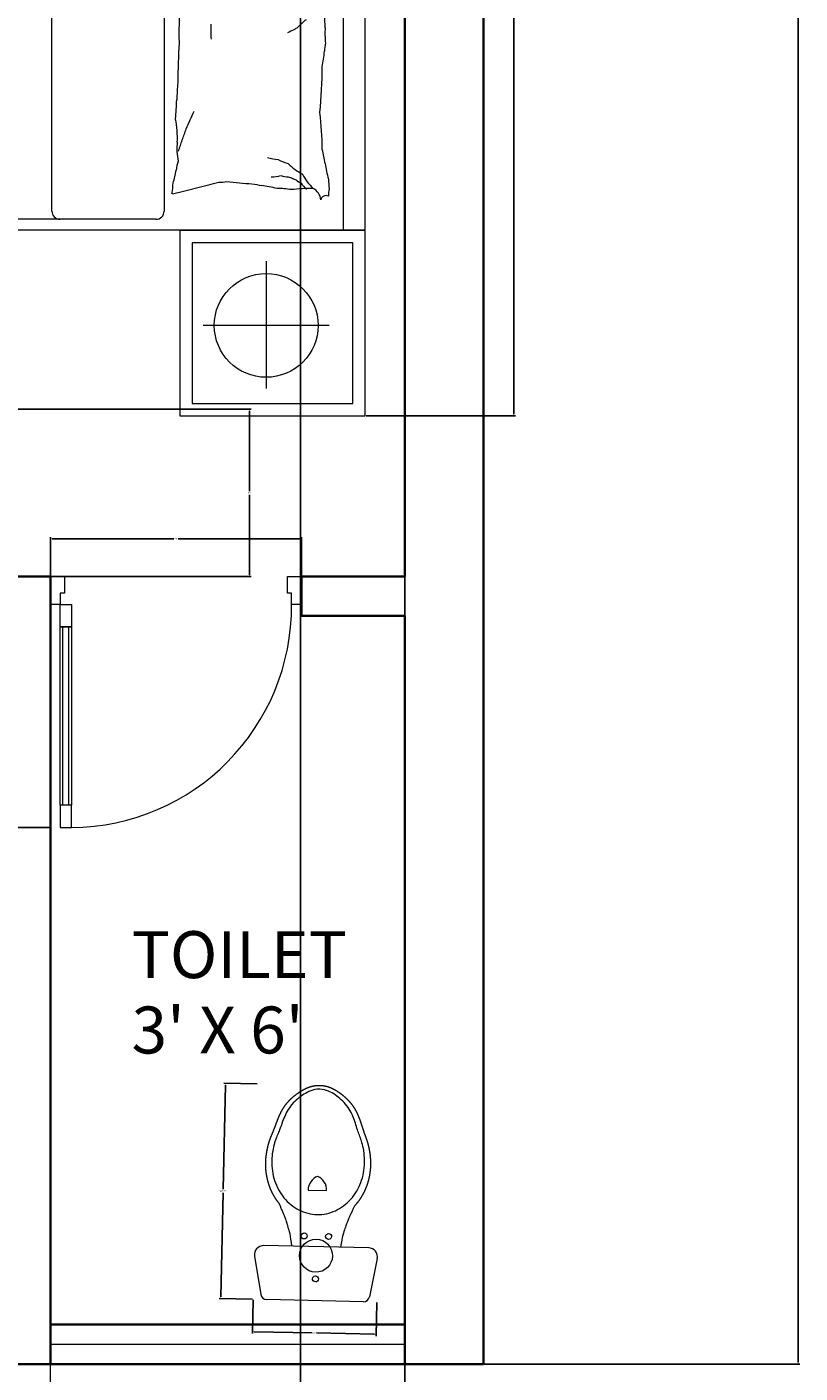
# Model space of a CAD drawing. Units: feet. Extents: x 1993 to 2298, y 2938 to 3641.
# Tile 4 of 11: x 2219 to 2298, y 3008 to 3144. Entities that reach past the tile are written whole.
import ezdxf

# ---------------------------------------------------------------- set-up
doc = ezdxf.new("R2010")
doc.units = ezdxf.units.FT
doc.linetypes.add('ACAD_ISO02W100', pattern=[15, 12, -3])
for name, color, linetype, lineweight in [('A-ANNO-DIMS', 2, 'Continuous', 18), ('A-AREA-IDEN', 7, 'Continuous', 18), ('A-DOOR', 3, 'Continuous', 18), ('A-FLOR-FIXT', 9, 'Continuous', 18), ('A-GLAZ', 4, 'Continuous', 13), ('DWV_RED', 7, 'Continuous', 0), ('furniture', 8, 'Continuous', 18), ('SUNSHADES', 4, 'ACAD_ISO02W100', 13), ('WAL', 7, 'Continuous', 35)]:
    doc.layers.add(name, color=color, linetype=linetype, lineweight=lineweight)
doc.styles.add('DIM_FONT', font='SIMPLEX.shx', dxfattribs={"width": 0.8})
doc.styles.get("Standard").update_dxf_attribs({"font": 'arial.ttf'})
doc.dimstyles.get("Standard").update_dxf_attribs({"dimtxt": 0.18, "dimasz": 0.18, "dimexe": 0.18, "dimexo": 0.0625, "dimgap": 0.09, "dimtad": 0, "dimtih": 1, "dimtoh": 1, "dimdec": 4, "dimzin": 0, "dimdsep": 46, "dimtxsty": 'Standard', "dimcen": 0.09, "dimadec": 0, "dimazin": 0, "dimtfac": 1, "dimtdec": 4, "dimtofl": 0, "dimtmove": 0, "dimatfit": 3, "dimfxl": 1, "dimtolj": 1, "dimtzin": 0, "dimarcsym": 0})

# ---------------------------------------------------------------- blocks, each defined once
blk = doc.blocks.new('A$C184E58E8')
for points in [[(825, 900), (825, 820), (865, 820), (865, 900)], [(825, 180), (825, 820), (865, 820), (865, 180)], [(835, 180), (835, 820), (855, 820), (855, 180)], [(825, 100), (825, 180), (865, 180), (865, 100)], [(35, 100), (35, 60), (50, 60), (50, 50), (50, 0), (0, 0), (0, 100)], [(865, 100), (900, 100), (900, 0), (850, 0), (850, 50), (850, 60), (865, 60)]]:
    blk.add_lwpolyline(points, close=True)
blk.add_arc((830, 105), 795, 90.3603, 180.3603)
blk = doc.blocks.new('A$C79766A75')
for p, q in [((1.9506, 2), (0.4506, 2)), ((1.9506, 0), (1.9506, 2)), ((2.402, 1.9999), (1.952, 1.9999)), ((1.952, 1.9999), (1.952, 1.5499)), ((2.402, 1.5499), (2.402, 1.9999)), ((2.372, 1.9699), (1.982, 1.9699)), ((1.982, 1.9699), (1.982, 1.5799)), ((2.372, 1.5799), (2.372, 1.9699)), ((1.9506, 1.9476), (0.4506, 1.9476)), ((2.1824, 1.9125), (2.1824, 1.6061)), ((2.0263, 1.7595), (2.3354, 1.7595)), ((1.8553, 1.5617), (1.8346, 1.6443)), ((1.982, 1.5799), (2.372, 1.5799)), ((1.8628, 1.5317), (1.8553, 1.5617)), ((1.952, 1.5499), (2.402, 1.5499)), ((1.0972, 1.5115), (1.9048, 1.5115)), ((1.9248, 1.4915), (1.9248, 0.0322)), ((1.9048, 1.2389), (1.0354, 1.2389))]:
    blk.add_line(p, q)
blk.add_circle((2.1824, 1.7595), 0.126)
for centre, radius, start, end in [((1.4683, 1.0293), 0.8732, 90.5757, 94.8018), ((1.4724, 2.1919), 0.2897, 267.4614, 274.8018), ((1.5236, 2.0532), 0.1524, 259.8101, 267.4614), ((1.4607, 1.3747), 0.5293, 79.8101, 83.9133), ((1.821, 1.6625), 0.2422, 97.5469, 105.744), ((1.7444, 2.2041), 0.3048, 278.4372, 285.744), ((1.8271, 2.0719), 0.1611, 270, 278.4372), ((1.8684, 2.0011), 0.0904, 258.7276, 270), ((1.8802, 1.9049), 0.0131, 153.4195, 258.7276), ((1.5543, 0.8466), 1.049, 83.9133, 90), ((1.7552, 1.2129), 0.6827, 90, 97.5469), ((1.7511, 1.9723), 0.1399, 297.2036, 314.9024), ((1.8802, 1.8579), 0.0342, 94.4002, 153.4195), ((2.3416, 1.8735), 0.4918, 180, 186.2324), ((1.615, 1.9982), 0.2252, 219.0349, 226.1885), ((1.5025, 1.8591), 0.0493, 208.3168, 219.0349), ((1.6908, 1.9123), 0.1399, 314.9024, 332.6012), ((1.6887, 1.8881), 0.1511, 334.6449, 338.1851), ((1.7896, 1.8667), 0.0526, 318.5571, 334.6449), ((1.784, 1.9167), 0.0899, 306.2641, 318.5571), ((1.6484, 1.9062), 0.2002, 203.0028, 208.3168), ((1.6554, 1.8529), 0.1399, 332.6012, 343.485), ((1.7653, 1.8132), 0.0562, 341.2201, 0), ((1.6307, 1.8895), 0.2056, 338.1851, 341.2201), ((2.0538, 1.7858), 0.204, 170.3156, 180), ((1.6404, 1.8023), 0.1399, 343.485, 354.3689), ((1.73, 1.7719), 0.0915, 0, 14.6851), ((2.7119, 1.5994), 0.882, 167.8016, 170.3156), ((1.5284, 1.792), 0.3171, 347.8016, 351.9949), ((1.1803, 1.7556), 0.6588, 351.9949, 357.3351), ((1.767, 1.6474), 0.0677, 357.3351, 14.0452), ((1.4679, 1.8969), 0.2721, 266.4448, 274.0828), ((1.3675, 0.9067), 0.7387, 64.6889, 66.5156), ((1.4107, 0.888), 0.7387, 66.5156, 68.3423), ((1.4677, 7.2662), 5.7185, 269.0296, 270.2865), ((1.6493, 4.9065), 3.3622, 267.3904, 269.0296), ((1.6903, 2.7573), 1.2165, 265.3824, 267.3904), ((1.5676, 0.139), 1.4048, 85.3824, 87.2509), ((1.7268, 1.3138), 0.2301, 87.2509, 101.5586), ((1.4594, 0.8688), 0.7387, 68.3423, 70.572), ((1.5136, 0.8497), 0.7387, 70.572, 72.8018), ((1.7541, 1.6886), 0.1459, 263.5659, 281.5586), ((1.8192, 1.6599), 0.1197, 252.6136, 263.5659), ((1.7679, 1.3144), 0.2297, 72.6136, 80.5159), ((1.8172, 1.2635), 0.2708, 80.5159, 85.9171), ((1.8627, 1.5308), 0.000917, 85.9171, 194.0449), ((1.9048, 1.4915), 0.02, 0, 90), ((1.9048, 1.2589), 0.02, 270, 0)]:
    blk.add_arc(centre, radius, start, end)
at = {"style": 'DIM_FONT', "text_generation_flag": 4, "width": 0.8, "flags": 9}
for tag in ['XSIZE', 'YSIZE']:
    blk.add_attdef(tag, (1.9506, 2), '', height=0.0005, rotation=180, dxfattribs=at)
blk = doc.blocks.new('A$C6F4D5F33')
at = {"layer": 'DWV_RED'}
for p, q in [((142.3, 403.6), (16.1, 380.5)), ((0, 42.9), (0, 361.2)), ((177.2, 29.5), (177.2, 374.6)), ((447.9, 353.8), (439.5, 353.3)), ((456.2, 354), (447.9, 353.8)), ((464.5, 353.9), (456.2, 354)), ((472.6, 353.4), (464.5, 353.9)), ((335.6, 311.2), (329.7, 305.8)), ((341.8, 316.3), (335.6, 311.2)), ((348.2, 321), (341.8, 316.3)), ((354.9, 325.5), (348.2, 321)), ((361.8, 329.7), (354.9, 325.5)), ((368.9, 333.5), (361.8, 329.7)), ((376.2, 337), (368.9, 333.5)), ((383.7, 340.2), (376.2, 337)), ((391.3, 343.1), (383.7, 340.2)), ((399.1, 345.6), (391.3, 343.1)), ((407, 347.8), (399.1, 345.6)), ((415, 349.7), (407, 347.8)), ((423.1, 351.2), (415, 349.7)), ((431.3, 352.5), (423.1, 351.2)), ((439.5, 353.3), (431.3, 352.5)), ((480.5, 352.6), (472.6, 353.4)), ((488.1, 351.6), (480.5, 352.6)), ((495.5, 350.4), (488.1, 351.6)), ((502.6, 349.1), (495.5, 350.4)), ((509.4, 347.5), (502.6, 349.1)), ((515.8, 345.9), (509.4, 347.5)), ((521.9, 344.1), (515.8, 345.9)), ((527.5, 342.3), (521.9, 344.1)), ((532.7, 340.4), (527.5, 342.3)), ((537.5, 338.6), (532.7, 340.4)), ((542, 336.9), (537.5, 338.6)), ((546.2, 335.2), (542, 336.9)), ((550.3, 333.5), (546.2, 335.2)), ((554.5, 331.9), (550.3, 333.5)), ((558.9, 330.3), (554.5, 331.9)), ((563.7, 328.6), (558.9, 330.3)), ((568.9, 326.8), (563.7, 328.6)), ((574.3, 324.9), (568.9, 326.8)), ((579.9, 323), (574.3, 324.9)), ((585.7, 321), (579.9, 323)), ((591.4, 318.9), (585.7, 321)), ((597.2, 316.8), (591.4, 318.9)), ((602.9, 314.5), (597.2, 316.8)), ((608.6, 312.1), (602.9, 314.5)), ((614.3, 309.5), (608.6, 312.1)), ((300.6, 268.4), (296.9, 261.5)), ((304.6, 275.2), (300.6, 268.4)), ((309, 281.8), (304.6, 275.2)), ((313.7, 288.1), (309, 281.8)), ((318.7, 294.3), (313.7, 288.1)), ((324, 300.1), (318.7, 294.3)), ((329.7, 305.8), (324, 300.1)), ((620, 306.6), (614.3, 309.5)), ((625.7, 303.4), (620, 306.6)), ((631.4, 299.9), (625.7, 303.4)), ((637, 296.1), (631.4, 299.9)), ((642.4, 291.8), (637, 296.1)), ((647.7, 287.3), (642.4, 291.8)), ((652.6, 282.7), (647.7, 287.3)), ((657.3, 277.9), (652.6, 282.7)), ((661.7, 273), (657.3, 277.9)), ((665.8, 268), (661.7, 273)), ((669.7, 263), (665.8, 268)), ((284.8, 224.5), (283.7, 216.9)), ((286.4, 232.1), (284.8, 224.5)), ((288.4, 239.6), (286.4, 232.1)), ((290.8, 247), (288.4, 239.6)), ((293.7, 254.3), (290.8, 247)), ((296.9, 261.5), (293.7, 254.3)), ((362.6, 232.5), (362.6, 171.6)), ((673.4, 258), (669.7, 263)), ((676.8, 253), (673.4, 258)), ((680.1, 247.8), (676.8, 253)), ((683.2, 242.5), (680.1, 247.8)), ((686.1, 236.7), (683.2, 242.5)), ((688.7, 230.6), (686.1, 236.7)), ((691.1, 224), (688.7, 230.6)), ((692.9, 217), (691.1, 224)), ((283.1, 209.2), (282.8, 201.5)), ((282.8, 201.5), (283.1, 193.8)), ((283.7, 216.9), (283.1, 209.2)), ((283.1, 193.8), (283.7, 186.1)), ((283.7, 186.1), (284.8, 178.4)), ((284.8, 178.4), (286.4, 170.8)), ((688.7, 172.4), (691.1, 179)), ((691.1, 179), (692.9, 186.1)), ((694.1, 209.4), (692.9, 217)), ((692.9, 186.1), (694.1, 193.6)), ((694.6, 201.5), (694.1, 209.4)), ((694.1, 193.6), (694.6, 201.5)), ((286.4, 170.8), (288.4, 163.3)), ((288.4, 163.3), (290.8, 155.9)), ((290.8, 155.9), (293.7, 148.6)), ((293.7, 148.6), (296.9, 141.5)), ((296.9, 141.5), (300.6, 134.5)), ((300.6, 134.5), (304.6, 127.7)), ((661.7, 130.1), (665.8, 135)), ((665.8, 135), (669.7, 140)), ((669.7, 140), (673.4, 145)), ((673.4, 145), (676.8, 150.1)), ((676.8, 150.1), (680.1, 155.2)), ((680.1, 155.2), (683.2, 160.6)), ((683.2, 160.6), (686.1, 166.3)), ((686.1, 166.3), (688.7, 172.4)), ((304.6, 127.7), (309, 121.2)), ((309, 121.2), (313.7, 114.8)), ((313.7, 114.8), (318.7, 108.7)), ((318.7, 108.7), (324, 102.8)), ((324, 102.8), (329.7, 97.2)), ((329.7, 97.2), (335.6, 91.8)), ((335.6, 91.8), (341.8, 86.7)), ((597.2, 86.3), (602.9, 88.6)), ((602.9, 88.6), (608.6, 91)), ((608.6, 91), (614.3, 93.6)), ((614.3, 93.6), (620, 96.4)), ((620, 96.4), (625.7, 99.6)), ((625.7, 99.6), (631.4, 103.1)), ((631.4, 103.1), (637, 107)), ((637, 107), (642.4, 111.2)), ((642.4, 111.2), (647.7, 115.7)), ((647.7, 115.7), (652.6, 120.4)), ((652.6, 120.4), (657.3, 125.2)), ((657.3, 125.2), (661.7, 130.1)), ((341.8, 86.7), (348.2, 81.9)), ((348.2, 81.9), (354.9, 77.4)), ((354.9, 77.4), (361.8, 73.3)), ((361.8, 73.3), (368.9, 69.4)), ((368.9, 69.4), (376.2, 65.9)), ((376.2, 65.9), (383.7, 62.7)), ((383.7, 62.7), (391.3, 59.8)), ((391.3, 59.8), (399.1, 57.3)), ((399.1, 57.3), (407, 55.1)), ((407, 55.1), (415, 53.2)), ((415, 53.2), (423.1, 51.7)), ((423.1, 51.7), (431.3, 50.5)), ((431.3, 50.5), (439.5, 49.6)), ((439.5, 49.6), (447.9, 49.1)), ((447.9, 49.1), (456.2, 48.9)), ((456.2, 48.9), (464.5, 49.1)), ((464.5, 49.1), (472.6, 49.6)), ((472.6, 49.6), (480.5, 50.3)), ((480.5, 50.3), (488.1, 51.3)), ((488.1, 51.3), (495.5, 52.5)), ((495.5, 52.5), (502.7, 53.9)), ((502.7, 53.9), (509.5, 55.4)), ((509.5, 55.4), (515.9, 57.1)), ((515.9, 57.1), (522, 58.9)), ((522, 58.9), (527.7, 60.8)), ((527.7, 60.8), (532.9, 62.6)), ((532.9, 62.6), (537.7, 64.5)), ((537.7, 64.5), (542.3, 66.2)), ((542.3, 66.2), (546.5, 68)), ((546.5, 68), (550.6, 69.6)), ((550.6, 69.6), (554.8, 71.2)), ((554.8, 71.2), (559.2, 72.8)), ((559.2, 72.8), (564, 74.5)), ((564, 74.5), (569.1, 76.3)), ((569.1, 76.3), (574.6, 78.2)), ((574.6, 78.2), (580.1, 80.1)), ((580.1, 80.1), (585.8, 82.1)), ((585.8, 82.1), (591.5, 84.2)), ((591.5, 84.2), (597.2, 86.3)), ((142.3, 0.5), (16.1, 23.6))]:
    blk.add_line(p, q, dxfattribs=at)
blk.add_lwpolyline([(177.2, 282.1), (189.7, 283.7), (200.3, 285.4), (209.4, 287.1), (217.2, 288.8), (223.8, 290.5), (229.5, 292.2), (234.5, 293.8), (239, 295.3), (243.3, 296.8), (247.4, 298.1), (251.3, 299.4), (254.9, 300.6), (258.4, 301.7), (261.7, 302.9), (264.8, 304), (267.8, 305.1), (270.6, 306.2), (273.3, 307.3), (275.9, 308.4), (278.5, 309.5), (281.1, 310.7), (283.7, 311.9), (286.3, 313.1), (289.1, 314.3), (291.9, 315.5), (294.8, 316.8), (297.7, 318), (300.5, 319.2), (303.3, 320.3), (305.8, 321.4), (308, 322.3), (310, 323.2), (311.5, 323.8), (312.8, 324.4), (313.8, 324.9), (314.6, 325.3), (315.2, 325.7), (315.7, 326), (316.2, 326.4), (316.7, 326.8), (317.3, 327.3), (318, 327.8), (318.7, 328.4), (319.5, 329), (320.3, 329.7), (321.1, 330.3), (322, 331), (322.9, 331.7), (323.8, 332.4), (324.7, 333.1), (325.6, 333.8), (326.5, 334.4), (327.4, 335.1), (328.3, 335.8), (329.2, 336.4), (330.1, 337.1), (331, 337.7), (331.9, 338.3), (332.9, 339), (333.8, 339.6), (334.7, 340.2), (335.7, 340.8), (336.6, 341.5), (337.6, 342.1), (338.5, 342.7), (339.5, 343.3), (340.4, 343.8), (341.4, 344.4), (342.3, 345), (343.3, 345.6), (344.3, 346.1), (345.2, 346.7), (346.2, 347.3), (347.2, 347.8), (348.2, 348.4), (349.2, 348.9), (350.2, 349.4), (351.1, 349.9), (352.1, 350.5), (353.1, 351), (354.1, 351.5), (355.1, 352), (356.2, 352.5), (357.2, 353), (358.2, 353.5), (359.2, 353.9), (360.2, 354.4), (361.2, 354.9), (362.3, 355.4), (363.3, 355.8), (364.3, 356.3), (365.4, 356.7), (366.4, 357.2), (367.4, 357.6), (368.5, 358), (369.5, 358.4), (370.6, 358.9), (371.6, 359.3), (372.7, 359.7), (373.7, 360.1), (374.8, 360.5), (375.8, 360.9), (376.9, 361.2), (378, 361.6), (379, 362), (380.1, 362.3), (381.2, 362.7), (382.3, 363.1), (383.3, 363.4), (384.4, 363.8), (385.5, 364.1), (386.6, 364.4), (387.7, 364.7), (388.7, 365.1), (389.8, 365.4), (390.9, 365.7), (392, 366), (393.1, 366.3), (394.2, 366.6), (395.3, 366.8), (396.4, 367.1), (397.5, 367.4), (398.6, 367.7), (399.7, 367.9), (400.8, 368.2), (401.9, 368.4), (403, 368.7), (404.1, 368.9), (405.2, 369.1), (406.3, 369.4), (407.4, 369.6), (408.5, 369.8), (409.7, 370), (410.8, 370.2), (411.9, 370.4), (413, 370.6), (414.1, 370.8), (415.3, 371), (416.4, 371.1), (417.5, 371.3), (418.6, 371.5), (419.8, 371.6), (420.9, 371.8), (422, 371.9), (423.1, 372.1), (424.3, 372.2), (425.4, 372.3), (426.5, 372.4), (427.7, 372.6), (428.8, 372.7), (429.9, 372.8), (431.1, 372.9), (432.2, 373), (433.4, 373.1), (434.5, 373.1), (435.6, 373.2), (436.8, 373.3), (437.9, 373.3), (439.1, 373.4), (440.2, 373.5), (441.4, 373.5), (442.5, 373.5), (443.6, 373.6), (444.8, 373.6), (445.9, 373.6), (447.1, 373.6), (448.2, 373.6), (449.3, 373.6), (450.5, 373.6), (451.6, 373.6), (452.8, 373.6), (453.9, 373.6), (455, 373.6), (456.1, 373.5), (457.3, 373.5), (458.4, 373.5), (459.5, 373.4), (460.6, 373.4), (461.7, 373.3), (462.8, 373.2), (463.9, 373.2), (465, 373.1), (466.1, 373), (467.2, 373), (468.3, 372.9), (469.4, 372.8), (470.5, 372.7), (471.5, 372.6), (472.6, 372.5), (473.7, 372.4), (474.7, 372.3), (475.8, 372.1), (476.8, 372), (477.9, 371.9), (478.9, 371.8), (480, 371.6), (481, 371.5), (482, 371.4), (483, 371.2), (484.1, 371.1), (485.1, 370.9), (486.1, 370.8), (487.1, 370.6), (488.1, 370.5), (489.1, 370.3), (490.1, 370.1), (491.1, 370), (492.1, 369.8), (493, 369.6), (494, 369.4), (495, 369.2), (495.9, 369.1), (496.9, 368.9), (497.8, 368.7), (498.8, 368.5), (499.7, 368.3), (500.7, 368.1), (501.6, 367.9), (502.5, 367.7), (503.5, 367.5), (504.4, 367.3), (505.3, 367.1), (506.2, 366.9), (507.1, 366.6), (508, 366.4), (508.9, 366.2), (509.8, 366), (510.7, 365.8), (511.5, 365.5), (512.4, 365.3), (513.3, 365.1), (514.1, 364.8), (515, 364.6), (515.8, 364.4), (516.7, 364.1), (517.5, 363.9), (518.3, 363.6), (519.1, 363.4), (519.9, 363.2), (520.7, 362.9), (521.5, 362.7), (522.3, 362.4), (523.1, 362.2), (523.9, 361.9), (524.6, 361.7), (525.4, 361.4), (526.1, 361.2), (526.9, 360.9), (527.6, 360.7), (528.3, 360.4), (529.1, 360.2), (529.8, 359.9), (530.5, 359.7), (531.2, 359.4), (531.9, 359.2), (532.5, 358.9), (533.2, 358.7), (533.9, 358.4), (534.5, 358.2), (535.2, 358), (535.8, 357.7), (536.4, 357.5), (537.1, 357.2), (537.7, 357), (538.3, 356.8), (538.9, 356.5), (539.5, 356.3), (540.1, 356.1), (540.6, 355.8), (541.2, 355.6), (541.8, 355.4), (542.3, 355.2), (542.9, 355), (543.4, 354.7), (544, 354.5), (544.5, 354.3), (545.1, 354.1), (545.6, 353.9), (546.1, 353.7), (546.6, 353.5), (547.1, 353.3), (547.6, 353.1), (548.2, 352.9), (548.7, 352.7), (549.2, 352.5), (549.6, 352.3), (550.1, 352.1), (550.6, 351.9), (551.1, 351.7), (551.6, 351.5), (552.1, 351.3), (552.6, 351.1), (553.1, 350.9), (553.6, 350.7), (554.1, 350.6), (554.6, 350.4), (555.1, 350.2), (555.6, 350), (556.1, 349.8), (556.7, 349.6), (557.2, 349.4), (557.7, 349.2), (558.3, 349), (558.8, 348.8), (559.4, 348.6), (560, 348.4), (560.5, 348.2), (561.1, 348), (561.7, 347.8), (562.3, 347.6), (562.9, 347.4), (563.5, 347.2), (564.1, 346.9), (564.7, 346.7), (565.4, 346.5), (566, 346.3), (566.6, 346.1), (567.3, 345.8), (567.9, 345.6), (568.6, 345.4), (569.2, 345.2), (569.9, 344.9), (570.6, 344.7), (571.2, 344.5), (571.9, 344.2), (572.6, 344), (573.3, 343.8), (574, 343.5), (574.7, 343.3), (575.4, 343), (576.1, 342.8), (576.8, 342.6), (577.5, 342.3), (578.2, 342.1), (578.9, 341.8), (579.6, 341.6), (580.3, 341.3), (581.1, 341.1), (581.8, 340.8), (582.5, 340.5), (583.3, 340.3), (584, 340), (584.7, 339.8), (585.4, 339.5), (586.2, 339.2), (586.9, 339), (587.7, 338.7), (588.4, 338.4), (589.1, 338.2), (589.9, 337.9), (590.6, 337.6), (591.4, 337.4), (592.1, 337.1), (592.9, 336.8), (593.6, 336.5), (594.4, 336.2), (595.1, 336), (595.9, 335.7), (596.6, 335.4), (597.4, 335.1), (598.2, 334.8), (598.9, 334.5), (599.7, 334.2), (600.4, 333.9), (601.2, 333.6), (602, 333.3), (602.7, 333), (603.5, 332.7), (604.3, 332.4), (605, 332.1), (605.8, 331.7), (606.6, 331.4), (607.3, 331.1), (608.1, 330.7), (608.9, 330.4), (609.7, 330.1), (610.5, 329.7), (611.2, 329.4), (612, 329), (612.8, 328.7), (613.6, 328.3), (614.4, 327.9), (615.2, 327.6), (616, 327.2), (616.8, 326.8), (617.6, 326.4), (618.4, 326), (619.2, 325.6), (620, 325.2), (620.8, 324.8), (621.6, 324.4), (622.4, 324), (623.2, 323.5), (624, 323.1), (624.8, 322.7), (625.6, 322.2), (626.4, 321.8), (627.2, 321.3), (628, 320.8), (628.8, 320.4), (629.6, 319.9), (630.4, 319.4), (631.2, 318.9), (632.1, 318.4), (632.9, 317.9), (633.7, 317.4), (634.5, 316.9), (635.3, 316.3), (636.1, 315.8), (636.9, 315.3), (637.7, 314.7), (638.5, 314.2), (639.3, 313.6), (640.1, 313.1), (640.9, 312.5), (641.7, 311.9), (642.5, 311.3), (643.3, 310.7), (644.1, 310.1), (644.9, 309.5), (645.7, 308.9), (646.4, 308.3), (647.2, 307.7), (648, 307.1), (648.7, 306.4), (649.5, 305.8), (650.3, 305.2), (651, 304.5), (651.8, 303.9), (652.5, 303.3), (653.2, 302.6), (654, 302), (654.7, 301.3), (655.4, 300.6), (656.1, 300), (656.8, 299.3), (657.5, 298.7), (658.2, 298), (658.9, 297.3), (659.6, 296.7), (660.2, 296), (660.9, 295.3), (661.6, 294.7), (662.2, 294), (662.9, 293.3), (663.5, 292.7), (664.2, 292), (664.8, 291.3), (665.4, 290.6), (666, 290), (666.7, 289.3), (667.3, 288.6), (667.9, 287.9), (668.5, 287.2), (669.1, 286.6), (669.7, 285.9), (670.3, 285.2), (670.9, 284.5), (671.4, 283.8), (672, 283.1), (672.6, 282.5), (673.2, 281.8), (673.7, 281.1), (674.3, 280.4), (674.8, 279.7), (675.4, 279), (675.9, 278.3), (676.5, 277.6), (677, 277), (677.5, 276.3), (678.1, 275.6), (678.6, 274.9), (679.1, 274.2), (679.6, 273.5), (680.1, 272.8), (680.6, 272.1), (681.1, 271.4), (681.6, 270.7), (682.1, 270), (682.6, 269.3), (683.1, 268.6), (683.6, 268), (684.1, 267.3), (684.5, 266.6), (685, 265.9), (685.5, 265.2), (686, 264.4), (686.4, 263.7), (686.9, 263), (687.4, 262.3), (687.8, 261.6), (688.3, 260.9), (688.7, 260.1), (689.2, 259.4), (689.6, 258.7), (690.1, 257.9), (690.5, 257.2), (691, 256.4), (691.4, 255.7), (691.9, 254.9), (692.3, 254.1), (692.7, 253.3), (693.2, 252.5), (693.6, 251.7), (694.1, 250.9), (694.5, 250.1), (694.9, 249.3), (695.3, 248.5), (695.8, 247.6), (696.2, 246.8), (696.6, 245.9), (697, 245), (697.4, 244.2), (697.8, 243.3), (698.2, 242.4), (698.6, 241.5), (699, 240.5), (699.4, 239.6), (699.8, 238.7), (700.2, 237.7), (700.6, 236.7), (700.9, 235.8), (701.3, 234.8), (701.6, 233.8), (702, 232.8), (702.3, 231.8), (702.7, 230.7), (703, 229.7), (703.3, 228.6), (703.6, 227.6), (703.9, 226.5), (704.2, 225.4), (704.5, 224.3), (704.7, 223.2), (705, 222.1), (705.2, 220.9), (705.5, 219.8), (705.7, 218.6), (705.9, 217.4), (706.1, 216.3), (706.3, 215.1), (706.4, 213.9), (706.6, 212.7), (706.7, 211.5), (706.9, 210.2), (707, 209), (707.1, 207.8), (707.1, 206.5), (707.2, 205.3), (707.2, 204), (707.3, 202.8), (707.3, 201.5), (707.3, 200.3), (707.2, 199), (707.2, 197.8), (707.1, 196.5), (707.1, 195.3), (707, 194), (706.9, 192.8), (706.7, 191.6), (706.6, 190.4), (706.4, 189.2), (706.3, 188), (706.1, 186.8), (705.9, 185.6), (705.7, 184.4), (705.5, 183.3), (705.2, 182.1), (705, 181), (704.7, 179.9), (704.5, 178.8), (704.2, 177.6), (703.9, 176.6), (703.6, 175.5), (703.3, 174.4), (703, 173.4), (702.7, 172.3), (702.3, 171.3), (702, 170.3), (701.6, 169.3), (701.3, 168.3), (700.9, 167.3), (700.6, 166.3), (700.2, 165.3), (699.8, 164.4), (699.4, 163.4), (699, 162.5), (698.6, 161.6), (698.2, 160.7), (697.8, 159.8), (697.4, 158.9), (697, 158), (696.6, 157.1), (696.2, 156.3), (695.8, 155.4), (695.3, 154.6), (694.9, 153.7), (694.5, 152.9), (694.1, 152.1), (693.6, 151.3), (693.2, 150.5), (692.7, 149.7), (692.3, 148.9), (691.9, 148.1), (691.4, 147.4), (691, 146.6), (690.5, 145.9), (690.1, 145.1), (689.6, 144.4), (689.2, 143.6), (688.7, 142.9), (688.3, 142.2), (687.8, 141.4), (687.4, 140.7), (686.9, 140), (686.4, 139.3), (686, 138.6), (685.5, 137.9), (685, 137.2), (684.5, 136.5), (684.1, 135.8), (683.6, 135.1), (683.1, 134.4), (682.6, 133.7), (682.1, 133), (681.6, 132.3), (681.1, 131.6), (680.6, 130.9), (680.1, 130.2), (679.6, 129.5), (679.1, 128.9), (678.6, 128.2), (678.1, 127.5), (677.5, 126.8), (677, 126.1), (676.5, 125.4), (675.9, 124.7), (675.4, 124), (674.8, 123.3), (674.3, 122.6), (673.7, 122), (673.2, 121.3), (672.6, 120.6), (672, 119.9), (671.4, 119.2), (670.9, 118.5), (670.3, 117.9), (669.7, 117.2), (669.1, 116.5), (668.5, 115.8), (667.9, 115.1), (667.3, 114.4), (666.7, 113.8), (666, 113.1), (665.4, 112.4), (664.8, 111.7), (664.2, 111.1), (663.5, 110.4), (662.9, 109.7), (662.2, 109), (661.6, 108.4), (660.9, 107.7), (660.2, 107), (659.6, 106.4), (658.9, 105.7), (658.2, 105), (657.5, 104.4), (656.8, 103.7), (656.1, 103.1), (655.4, 102.4), (654.7, 101.7), (654, 101.1), (653.2, 100.4), (652.5, 99.8), (651.8, 99.1), (651, 98.5), (650.3, 97.9), (649.5, 97.2), (648.7, 96.6), (648, 96), (647.2, 95.3), (646.4, 94.7), (645.7, 94.1), (644.9, 93.5), (644.1, 92.9), (643.3, 92.3), (642.5, 91.7), (641.7, 91.1), (640.9, 90.6), (640.1, 90), (639.3, 89.4), (638.5, 88.9), (637.7, 88.3), (636.9, 87.8), (636.1, 87.2), (635.3, 86.7), (634.5, 86.2), (633.7, 85.7), (632.9, 85.1), (632.1, 84.6), (631.3, 84.1), (630.4, 83.7), (629.6, 83.2), (628.8, 82.7), (628, 82.2), (627.2, 81.8), (626.4, 81.3), (625.6, 80.8), (624.8, 80.4), (624, 80), (623.2, 79.5), (622.4, 79.1), (621.6, 78.7), (620.8, 78.3), (620, 77.8), (619.2, 77.4), (618.4, 77), (617.6, 76.7), (616.8, 76.3), (616, 75.9), (615.2, 75.5), (614.4, 75.1), (613.6, 74.8), (612.8, 74.4), (612.1, 74), (611.3, 73.7), (610.5, 73.3), (609.7, 73), (608.9, 72.7), (608.2, 72.3), (607.4, 72), (606.6, 71.7), (605.8, 71.3), (605.1, 71), (604.3, 70.7), (603.5, 70.4), (602.8, 70.1), (602, 69.8), (601.3, 69.5), (600.5, 69.1), (599.7, 68.9), (599, 68.6), (598.2, 68.3), (597.5, 68), (596.7, 67.7), (596, 67.4), (595.2, 67.1), (594.5, 66.8), (593.7, 66.5), (593, 66.3), (592.2, 66), (591.5, 65.7), (590.7, 65.4), (590, 65.2), (589.3, 64.9), (588.5, 64.6), (587.8, 64.4), (587, 64.1), (586.3, 63.8), (585.6, 63.6), (584.8, 63.3), (584.1, 63.1), (583.4, 62.8), (582.7, 62.5), (581.9, 62.3), (581.2, 62), (580.5, 61.8), (579.8, 61.5), (579.1, 61.3), (578.4, 61), (577.7, 60.8), (577, 60.6), (576.3, 60.3), (575.6, 60.1), (574.9, 59.8), (574.2, 59.6), (573.5, 59.4), (572.8, 59.1), (572.1, 58.9), (571.5, 58.7), (570.8, 58.4), (570.1, 58.2), (569.5, 58), (568.8, 57.7), (568.2, 57.5), (567.5, 57.3), (566.9, 57.1), (566.2, 56.8), (565.6, 56.6), (565, 56.4), (564.4, 56.2), (563.8, 56), (563.2, 55.8), (562.6, 55.5), (562, 55.3), (561.4, 55.1), (560.8, 54.9), (560.2, 54.7), (559.7, 54.5), (559.1, 54.3), (558.6, 54.1), (558, 53.9), (557.5, 53.7), (557, 53.5), (556.5, 53.3), (555.9, 53.1), (555.4, 53), (554.9, 52.8), (554.4, 52.6), (553.9, 52.4), (553.4, 52.2), (552.9, 52), (552.4, 51.8), (551.9, 51.6), (551.5, 51.4), (551, 51.2), (550.5, 51.1), (550, 50.9), (549.5, 50.7), (549, 50.5), (548.5, 50.3), (548, 50.1), (547.5, 49.9), (546.9, 49.7), (546.4, 49.4), (545.9, 49.2), (545.4, 49), (544.8, 48.8), (544.3, 48.6), (543.8, 48.4), (543.2, 48.2), (542.6, 47.9), (542.1, 47.7), (541.5, 47.5), (540.9, 47.3), (540.4, 47), (539.8, 46.8), (539.2, 46.6), (538.6, 46.3), (538, 46.1), (537.3, 45.9), (536.7, 45.6), (536.1, 45.4), (535.4, 45.1), (534.8, 44.9), (534.1, 44.6), (533.5, 44.4), (532.8, 44.1), (532.1, 43.9), (531.4, 43.6), (530.7, 43.4), (530, 43.1), (529.3, 42.9), (528.6, 42.6), (527.8, 42.4), (527.1, 42.1), (526.4, 41.9), (525.6, 41.6), (524.8, 41.4), (524.1, 41.1), (523.3, 40.9), (522.5, 40.6), (521.7, 40.4), (520.9, 40.1), (520.1, 39.9), (519.3, 39.6), (518.5, 39.4), (517.7, 39.1), (516.8, 38.9), (516, 38.6), (515.1, 38.4), (514.3, 38.2), (513.4, 37.9), (512.5, 37.7), (511.7, 37.5), (510.8, 37.2), (509.9, 37), (509, 36.8), (508.1, 36.6), (507.2, 36.3), (506.3, 36.1), (505.4, 35.9), (504.5, 35.7), (503.6, 35.5), (502.6, 35.3), (501.7, 35.1), (500.8, 34.9), (499.8, 34.7), (498.9, 34.5), (497.9, 34.3), (497, 34.1), (496, 33.9), (495, 33.7), (494.1, 33.5), (493.1, 33.4), (492.1, 33.2), (491.1, 33), (490.1, 32.8), (489.1, 32.7), (488.1, 32.5), (487.1, 32.3), (486.1, 32.2), (485.1, 32), (484.1, 31.9), (483.1, 31.7), (482.1, 31.6), (481, 31.4), (480, 31.3), (478.9, 31.2), (477.9, 31.1), (476.9, 30.9), (475.8, 30.8), (474.7, 30.7), (473.7, 30.6), (472.6, 30.5), (471.6, 30.4), (470.5, 30.3), (469.4, 30.2), (468.3, 30.1), (467.2, 30), (466.1, 29.9), (465, 29.8), (463.9, 29.8), (462.8, 29.7), (461.7, 29.6), (460.6, 29.6), (459.5, 29.5), (458.4, 29.5), (457.3, 29.4), (456.1, 29.4), (455, 29.4), (453.9, 29.3), (452.8, 29.3), (451.6, 29.3), (450.5, 29.3), (449.3, 29.3), (448.2, 29.3), (447.1, 29.3), (445.9, 29.3), (444.8, 29.3), (443.6, 29.4), (442.5, 29.4), (441.4, 29.4), (440.2, 29.5), (439.1, 29.5), (437.9, 29.6), (436.8, 29.7), (435.6, 29.7), (434.5, 29.8), (433.4, 29.9), (432.2, 30), (431.1, 30.1), (429.9, 30.2), (428.8, 30.3), (427.7, 30.4), (426.5, 30.5), (425.4, 30.6), (424.3, 30.7), (423.1, 30.9), (422, 31), (420.9, 31.2), (419.8, 31.3), (418.6, 31.5), (417.5, 31.6), (416.4, 31.8), (415.3, 32), (414.1, 32.2), (413, 32.3), (411.9, 32.5), (410.8, 32.7), (409.7, 32.9), (408.5, 33.1), (407.4, 33.4), (406.3, 33.6), (405.2, 33.8), (404.1, 34), (403, 34.3), (401.9, 34.5), (400.8, 34.8), (399.7, 35), (398.6, 35.3), (397.5, 35.5), (396.4, 35.8), (395.3, 36.1), (394.2, 36.4), (393.1, 36.7), (392, 37), (390.9, 37.3), (389.8, 37.6), (388.7, 37.9), (387.7, 38.2), (386.6, 38.5), (385.5, 38.9), (384.4, 39.2), (383.3, 39.5), (382.3, 39.9), (381.2, 40.2), (380.1, 40.6), (379, 41), (378, 41.3), (376.9, 41.7), (375.8, 42.1), (374.8, 42.5), (373.7, 42.9), (372.7, 43.3), (371.6, 43.7), (370.6, 44.1), (369.5, 44.5), (368.5, 44.9), (367.4, 45.4), (366.4, 45.8), (365.4, 46.2), (364.3, 46.7), (363.3, 47.1), (362.3, 47.6), (361.2, 48), (360.2, 48.5), (359.2, 49), (358.2, 49.5), (357.2, 50), (356.2, 50.5), (355.1, 50.9), (354.1, 51.5), (353.1, 52), (352.1, 52.5), (351.1, 53), (350.2, 53.5), (349.2, 54.1), (348.2, 54.6), (347.2, 55.1), (346.2, 55.7), (345.2, 56.2), (344.3, 56.8), (343.3, 57.4), (342.3, 57.9), (341.4, 58.5), (340.4, 59.1), (339.5, 59.7), (338.5, 60.3), (337.6, 60.9), (336.6, 61.5), (335.7, 62.1), (334.7, 62.7), (333.8, 63.3), (332.9, 64), (331.9, 64.6), (331, 65.2), (330.1, 65.9), (329.2, 66.5), (328.3, 67.2), (327.4, 67.8), (326.5, 68.5), (325.6, 69.2), (324.7, 69.9), (323.8, 70.5), (322.9, 71.2), (322, 71.9), (321.1, 72.6), (320.3, 73.3), (319.5, 74), (318.7, 74.6), (317.9, 75.3), (317.2, 75.9), (316.5, 76.4), (315.9, 76.9), (315.3, 77.4), (314.6, 77.9), (313.9, 78.5), (313, 79), (311.9, 79.6), (310.6, 80.3), (309, 81.1), (307.1, 82), (304.9, 82.9), (302.5, 84), (299.9, 85.1), (297.2, 86.3), (294.4, 87.5), (291.6, 88.7), (288.8, 89.9), (286.2, 91.1), (283.6, 92.3), (281, 93.4), (278.5, 94.6), (275.9, 95.7), (273.3, 96.8), (270.6, 97.9), (267.8, 99), (264.8, 100.1), (261.7, 101.2), (258.4, 102.4), (254.9, 103.5), (251.3, 104.7), (247.4, 106), (243.3, 107.3), (239, 108.8), (234.5, 110.3), (229.5, 111.9), (223.8, 113.6), (217.2, 115.3), (209.4, 117), (200.3, 118.7), (189.7, 120.4), (177.2, 122)], dxfattribs=at)
for centre, major_axis, start_param, end_param in [((147.6, 374.6), (-20.9, 20.9), 3.926991, 5.678651), ((19.7, 361.2), (-13.9, 13.9), 5.678651, 7.068583), ((147.6, 202.1), (-38.3, 38.3), 0.785398, 7.068583), ((211.6, 242.1), (-6.96, 6.96), 0.785398, 7.068583), ((362.6, 182.9), (-35.1, -35.1), 2.753037, 3.926991), ((71.5, 202.2), (-6.96, -6.96), -0.785398, 5.497787), ((362.6, 221.2), (-35.1, 35.1), 2.356194, 3.530149), ((211.6, 162), (-6.96, 6.96), 0.785398, 7.068583), ((19.7, 42.9), (-13.9, -13.9), -0.785398, 0.604534), ((147.6, 29.5), (-20.9, -20.9), 0.604534, 2.356194)]:
    blk.add_ellipse(centre, major_axis=major_axis, ratio=1, start_param=start_param, end_param=end_param, dxfattribs=at)
blk = doc.blocks.new('*D28')
at = {"layer": 'A-ANNO-DIMS', "color": 0, "lineweight": -2, "transparency": 16777216}
for p, q in [((2221.7, 3088.53), (2217.75, 3088.53)), ((2217.93, 3088.35), (2217.93, 3075.97)), ((2217.93, 3063.22), (2217.93, 3075.6)), ((2221.7, 3063.04), (2217.75, 3063.04))]:
    blk.add_line(p, q, dxfattribs=at)
at = {"layer": 'A-ANNO-DIMS', "color": 0, "transparency": 16777216}
for points in [[(2217.9, 3088.35), (2217.96, 3088.35), (2217.93, 3088.53)], [(2217.9, 3063.22), (2217.96, 3063.22), (2217.93, 3063.04)]]:
    blk.add_solid(points, dxfattribs=at)
at = {"layer": 'Defpoints', "color": 0, "transparency": 16777216}
for p in [(2221.76, 3088.53), (2217.93, 3063.04), (2221.76, 3063.04)]:
    blk.add_point(p, dxfattribs=at)
at = {"layer": 'A-ANNO-DIMS', "color": 0, "transparency": 16777216, "insert": (2217.93, 3075.78), "char_height": 0.18, "attachment_point": 5}
blk.add_mtext('\\A1;DOOR 25', dxfattribs=at)
blk = doc.blocks.new('*D29')
at = {"layer": 'A-ANNO-DIMS', "color": 0, "lineweight": -2, "transparency": 16777216}
for p, q in [((2221.76, 3088.6), (2221.76, 3092.54)), ((2221.94, 3092.36), (2234.29, 3092.36)), ((2247.08, 3092.36), (2234.73, 3092.36)), ((2247.26, 3088.6), (2247.26, 3092.54))]:
    blk.add_line(p, q, dxfattribs=at)
at = {"layer": 'A-ANNO-DIMS', "color": 0, "transparency": 16777216}
for points in [[(2221.94, 3092.39), (2221.94, 3092.33), (2221.76, 3092.36)], [(2247.08, 3092.39), (2247.08, 3092.33), (2247.26, 3092.36)]]:
    blk.add_solid(points, dxfattribs=at)
at = {"layer": 'Defpoints', "color": 0, "transparency": 16777216}
for p in [(2221.76, 3092.36), (2221.76, 3088.53), (2247.26, 3088.53)]:
    blk.add_point(p, dxfattribs=at)
at = {"layer": 'A-ANNO-DIMS', "color": 0, "transparency": 16777216, "insert": (2234.51, 3092.36), "char_height": 0.18, "attachment_point": 5}
blk.add_mtext('\\A1;25', dxfattribs=at)
blk = doc.blocks.new('*D30')
at = {"layer": 'A-ANNO-DIMS', "color": 0, "lineweight": -2, "transparency": 16777216}
for p, q in [((2253.83, 3205.36), (2269.02, 3205.36)), ((2268.84, 3205.18), (2268.84, 3155.29)), ((2268.84, 3105.04), (2268.84, 3154.93)), ((2253.83, 3104.86), (2269.02, 3104.86))]:
    blk.add_line(p, q, dxfattribs=at)
at = {"layer": 'A-ANNO-DIMS', "color": 0, "transparency": 16777216}
for points in [[(2268.81, 3205.18), (2268.87, 3205.18), (2268.84, 3205.36)], [(2268.81, 3105.04), (2268.87, 3105.04), (2268.84, 3104.86)]]:
    blk.add_solid(points, dxfattribs=at)
at = {"layer": 'Defpoints', "color": 0, "transparency": 16777216}
for p in [(2253.76, 3205.36), (2253.76, 3104.86), (2268.84, 3104.86)]:
    blk.add_point(p, dxfattribs=at)
at = {"layer": 'A-ANNO-DIMS', "color": 0, "transparency": 16777216, "insert": (2268.84, 3155.11), "char_height": 0.18, "attachment_point": 5}
blk.add_mtext('\\A1;BED & NIGHTSTANDS 100 TYP.', dxfattribs=at)
blk = doc.blocks.new('*D34')
at = {"layer": 'A-ANNO-DIMS', "color": 0, "lineweight": -2, "transparency": 16777216}
for p, q in [((2239.54, 3036.88), (2239.31, 3026.3)), ((2242.77, 3036.99), (2239.37, 3037.06)), ((2239.08, 3015.36), (2239.31, 3025.93)), ((2242.29, 3015.11), (2238.9, 3015.18))]:
    blk.add_line(p, q, dxfattribs=at)
at = {"layer": 'A-ANNO-DIMS', "color": 0, "transparency": 16777216}
for points in [[(2239.51, 3036.88), (2239.57, 3036.88), (2239.55, 3037.06)], [(2239.05, 3015.36), (2239.11, 3015.36), (2239.08, 3015.18)]]:
    blk.add_solid(points, dxfattribs=at)
at = {"layer": 'Defpoints', "color": 0, "transparency": 16777216}
for p in [(2239.55, 3037.06), (2242.83, 3036.99), (2242.36, 3015.11)]:
    blk.add_point(p, dxfattribs=at)
at = {"layer": 'A-ANNO-DIMS', "color": 0, "transparency": 16777216, "insert": (2239.31, 3026.12), "char_height": 0.18, "attachment_point": 5}
blk.add_mtext('\\A1;WC 22', dxfattribs=at)
blk = doc.blocks.new('*D35')
at = {"layer": 'A-ANNO-DIMS', "color": 0, "lineweight": -2, "transparency": 16777216}
for p, q in [((2242.36, 3015.05), (2242.28, 3011.65)), ((2254.92, 3014.78), (2254.85, 3011.38)), ((2242.47, 3011.82), (2248.36, 3011.7)), ((2254.67, 3011.56), (2248.78, 3011.69))]:
    blk.add_line(p, q, dxfattribs=at)
at = {"layer": 'A-ANNO-DIMS', "color": 0, "transparency": 16777216}
for points in [[(2242.47, 3011.85), (2242.47, 3011.79), (2242.29, 3011.83)], [(2254.67, 3011.59), (2254.67, 3011.53), (2254.85, 3011.56)]]:
    blk.add_solid(points, dxfattribs=at)
at = {"layer": 'Defpoints', "color": 0, "transparency": 16777216}
for p in [(2242.36, 3015.11), (2254.92, 3014.84), (2242.29, 3011.83)]:
    blk.add_point(p, dxfattribs=at)
at = {"layer": 'A-ANNO-DIMS', "color": 0, "transparency": 16777216, "insert": (2248.57, 3011.69), "char_height": 0.18, "attachment_point": 5}
blk.add_mtext('\\A1;13', dxfattribs=at)
blk = doc.blocks.new('*D55')
at = {"layer": 'A-ANNO-DIMS', "color": 0, "lineweight": -2, "transparency": 16777216}
for p, q in [((2265.82, 3608.53), (2297.9, 3608.53)), ((2297.72, 3608.35), (2297.72, 3308.72)), ((2297.72, 3008.71), (2297.72, 3308.35)), ((2265.82, 3008.53), (2297.9, 3008.53))]:
    blk.add_line(p, q, dxfattribs=at)
at = {"layer": 'A-ANNO-DIMS', "color": 0, "transparency": 16777216}
for points in [[(2297.69, 3608.35), (2297.75, 3608.35), (2297.72, 3608.53)], [(2297.69, 3008.71), (2297.75, 3008.71), (2297.72, 3008.53)]]:
    blk.add_solid(points, dxfattribs=at)
at = {"layer": 'Defpoints', "color": 0, "transparency": 16777216}
for p in [(2265.76, 3608.53), (2297.72, 3608.53), (2265.76, 3008.53)]:
    blk.add_point(p, dxfattribs=at)
at = {"layer": 'A-ANNO-DIMS', "color": 0, "transparency": 16777216, "insert": (2297.72, 3308.53), "char_height": 0.18, "attachment_point": 5}
blk.add_mtext('\\A1;600', dxfattribs=at)
blk = doc.blocks.new('*D66')
at = {"layer": 'A-ANNO-DIMS', "color": 0, "lineweight": -2, "transparency": 16777216}
for p, q in [((2247.15, 3235.34), (2247.15, 2937.86)), ((2257.76, 3228.47), (2257.76, 2937.86)), ((2247.33, 2938.03), (2252, 2938.03)), ((2257.58, 2938.03), (2252.91, 2938.03))]:
    blk.add_line(p, q, dxfattribs=at)
at = {"layer": 'A-ANNO-DIMS', "color": 0, "transparency": 16777216}
for points in [[(2247.33, 2938.07), (2247.33, 2938.01), (2247.15, 2938.03)], [(2257.58, 2938.07), (2257.58, 2938.01), (2257.76, 2938.03)]]:
    blk.add_solid(points, dxfattribs=at)
at = {"layer": 'Defpoints', "color": 0, "transparency": 16777216}
for p in [(2247.15, 3235.4), (2257.76, 3228.53), (2257.76, 2938.03)]:
    blk.add_point(p, dxfattribs=at)
at = {"layer": 'A-ANNO-DIMS', "color": 0, "transparency": 16777216, "insert": (2252.45, 2938.03), "char_height": 0.18, "attachment_point": 5}
blk.add_mtext('\\A1;10.608', dxfattribs=at)
blk = doc.blocks.new('*D74')
at = {"layer": 'A-ANNO-DIMS', "color": 0, "lineweight": -2, "transparency": 16777216}
for p, q in [((2210.06, 3105.53), (2242.15, 3105.53)), ((2241.97, 3105.35), (2241.97, 3097.21)), ((2241.97, 3088.71), (2241.97, 3096.85)), ((2210.06, 3088.53), (2242.15, 3088.53))]:
    blk.add_line(p, q, dxfattribs=at)
at = {"layer": 'A-ANNO-DIMS', "color": 0, "transparency": 16777216}
for points in [[(2241.94, 3105.35), (2242, 3105.35), (2241.97, 3105.53)], [(2241.94, 3088.71), (2242, 3088.71), (2241.97, 3088.53)]]:
    blk.add_solid(points, dxfattribs=at)
at = {"layer": 'Defpoints', "color": 0, "transparency": 16777216}
for p in [(2210, 3105.53), (2210, 3088.53), (2241.97, 3088.53)]:
    blk.add_point(p, dxfattribs=at)
at = {"layer": 'A-ANNO-DIMS', "color": 0, "transparency": 16777216, "insert": (2241.97, 3097.03), "char_height": 0.18, "attachment_point": 5}
blk.add_mtext('\\A1;17', dxfattribs=at)

msp = doc.modelspace()

# ---------------------------------------------------------------- linework, layer by layer
at = {"layer": 'A-GLAZ'}
msp.add_line((2257.7583, 3010.5338), (2221.7583, 3010.5338), dxfattribs=at)
at = {"layer": 'SUNSHADES'}
msp.add_line((2221.7583, 2970), (2221.7583, 3010.5338), dxfattribs=at)
at = {"layer": 'WAL'}
for p, q in [((2265.7583, 3608.5338), (2265.7583, 3008.5338)), ((2257.7583, 3224.5338), (2257.7583, 3088.5338)), ((2149.7583, 3088.5338), (2221.7583, 3088.5338)), ((2221.7583, 3084.5338), (2221.7583, 3088.5338)), ((2247.256, 3088.5338), (2247.256, 3084.5338)), ((2247.256, 3088.5338), (2257.7583, 3088.5338)), ((2221.7583, 3084.5338), (2221.7583, 3008.5338)), ((2247.256, 3084.5338), (2257.7583, 3084.5338)), ((2257.7583, 3084.5338), (2257.7583, 3008.5338)), ((2257.7583, 3012.5338), (2221.7583, 3012.5338)), ((2265.7583, 3008.5338), (2140, 3008.5338))]:
    msp.add_line(p, q, dxfattribs=at)

# ---------------------------------------------------------------- block references
at = {"layer": 'A-DOOR', "xscale": 0.0283306926372799, "yscale": 0.0283306926372799, "zscale": 0.0283306926372799, "rotation": 180}
msp.add_blockref('A$C184E58E8', (2247.256, 3088.5338), dxfattribs=at)
at = {"layer": 'A-FLOR-FIXT', "xscale": 0.0309308513494672, "yscale": 0.0309308513494672, "zscale": 0.0309308513494672, "rotation": 88.76557468731332}
msp.add_blockref('A$C6F4D5F33', (2254.8869, 3014.8382), dxfattribs=at)
at = {"layer": 'furniture', "xscale": 41.83725109546206, "yscale": 41.83725109546206, "zscale": 41.83725109546206, "rotation": 270}
msp.add_blockref('A$C79766A75', (2170.0686, 3205.3572), dxfattribs=at)

# ---------------------------------------------------------------- texts
at = {"layer": 'A-AREA-IDEN'}
for s, p in [('TOILET', (2230, 3047.7424)), ("3' X 6'", (2230, 3040.0845))]:
    msp.add_text(s, height=4.76705, dxfattribs=at).set_placement(p)

# ---------------------------------------------------------------- dimensions: what is measured, and where the dimension line sits
at = {"layer": 'A-ANNO-DIMS'}
for base, p1, p2, angle, picture, middle in [((2297.7233, 3608.5338), (2265.7583, 3008.5338), (2265.7583, 3608.5338), 90, '*D55', (2297.7233, 3308.5338)), ((2241.965, 3088.5338), (2210, 3105.5338), (2210, 3088.5338), 270, '*D74', (2241.965, 3097.0338)), ((2221.7583, 3092.3584), (2247.256, 3088.5338), (2221.7583, 3088.5338), 180, '*D29', (2234.5071, 3092.3584)), ((2242.2859, 3011.8266), (2254.9208, 3014.8375), (2242.3567, 3015.1082), 178.765575, '*D35', (2248.568, 3011.6913))]:
    dim = msp.add_linear_dim(base=base, p1=p1, p2=p2, angle=angle, dimstyle='Standard', override={"dimdec": 0, "dimlfac": 1, "dimrnd": 0, "dimzin": 0, "dimdsep": 46, "dimlunit": 2}, dxfattribs=at)
    dim.commit()
    dim.dimension.update_dxf_attribs({"geometry": picture, "text_midpoint": middle})
dim = msp.add_linear_dim(base=(2257.7583, 2938.035), p1=(2247.1506, 3235.4), p2=(2257.7583, 3228.5338), dimstyle='Standard', override={"dimdec": 3, "dimlfac": 1, "dimrnd": 0, "dimzin": 0, "dimdsep": 46, "dimlunit": 2}, dxfattribs=at)
dim.commit()
dim.dimension.update_dxf_attribs({"geometry": '*D66', "text_midpoint": (2252.4545, 2938.035)})
for base, p1, p2, angle, text, picture, middle in [((2268.8379, 3104.8648), (2253.764, 3205.3572), (2253.764, 3104.8648), 270, 'BED & NIGHTSTANDS <> TYP.', '*D30', (2268.8379, 3155.111)), ((2217.9337, 3063.0362), (2221.7583, 3088.5338), (2221.7583, 3063.0362), 270, 'DOOR <>', '*D28', (2217.9337, 3075.785)), ((2239.5465, 3037.0562), (2242.3567, 3015.1082), (2242.8281, 3036.9855), 88.765575, 'WC <>', '*D34', (2239.3108, 3026.1176))]:
    dim = msp.add_linear_dim(base=base, p1=p1, p2=p2, angle=angle, text=text, dimstyle='Standard', override={"dimdec": 0, "dimlfac": 1, "dimrnd": 0, "dimzin": 0, "dimdsep": 46, "dimlunit": 2}, dxfattribs=at)
    dim.commit()
    dim.dimension.update_dxf_attribs({"geometry": picture, "text_midpoint": middle})

doc.saveas('drawing.dxf')
